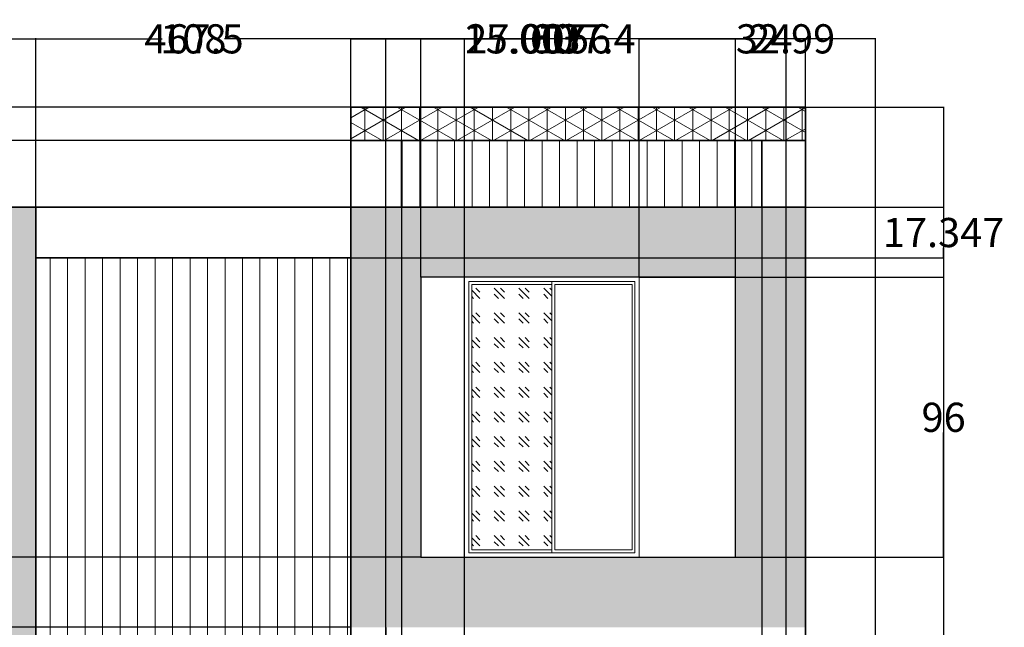
# Model space of a CAD drawing. Units: inches. Extents: x -37 to 519, y -28 to 435.
# Tile 3 of 3: x 182 to 519, y 227 to 435. Entities that reach past the tile are written whole.
import ezdxf

# ---------------------------------------------------------------- set-up
doc = ezdxf.new("R2010")
doc.units = ezdxf.units.IN
doc.header["$MEASUREMENT"] = 0
for name, color, linetype, lineweight in [('A-ANNO-DIMS', 2, 'Continuous', 18), ('A-GLAZ', 4, 'Continuous', 18), ('A-GLAZ-PATT', 9, 'Continuous', 13), ('A-ROOF', 7, 'Continuous', 35), ('A-ROOF-PATT', 8, 'Continuous', 13), ('A-WALL', 7, 'Continuous', 35), ('A-WALL-PATT', 8, 'Continuous', 13), ('A-WALL-TRIM', 7, 'Continuous', 25)]:
    doc.layers.add(name, color=color, linetype=linetype, lineweight=lineweight)
doc.styles.get("Standard").update_dxf_attribs({"font": 'arial.ttf'})
doc.dimstyles.get("Standard").update_dxf_attribs({"dimtxt": 10, "dimasz": 0.18, "dimexe": 0.18, "dimexo": 0.0625, "dimgap": 0.09, "dimtad": 0, "dimtih": 1, "dimtoh": 1, "dimdec": 0, "dimzin": 0, "dimdsep": 46, "dimlunit": 3, "dimtxsty": 'Standard', "dimcen": 0.09, "dimadec": 0, "dimazin": 0, "dimtfac": 1, "dimtdec": 0, "dimtofl": 0, "dimtmove": 0, "dimatfit": 3, "dimfxl": 1, "dimtolj": 1, "dimtzin": 0, "dimarcsym": 0})

# ---------------------------------------------------------------- blocks, each defined once
blk = doc.blocks.new('*D7')
at = {"layer": 'A-ANNO-DIMS', "color": 0, "lineweight": -2, "transparency": 16777216}
for p, q in [((7.62, 97.72), (7.62, 428.56)), ((7.8, 428.38), (224.17, 428.38)), ((474.95, 428.38), (258.57, 428.38)), ((475.13, 97.72), (475.13, 428.56))]:
    blk.add_line(p, q, dxfattribs=at)
at = {"layer": 'A-ANNO-DIMS', "color": 0, "transparency": 16777216}
for points in [[(7.8, 428.41), (7.8, 428.35), (7.62, 428.38)], [(474.95, 428.41), (474.95, 428.35), (475.13, 428.38)]]:
    blk.add_solid(points, dxfattribs=at)
at = {"layer": 'Defpoints', "color": 0, "transparency": 16777216}
for p in [(475.13, 428.38), (7.62, 97.65), (475.13, 97.65)]:
    blk.add_point(p, dxfattribs=at)
at = {"layer": 'A-ANNO-DIMS', "color": 0, "transparency": 16777216, "insert": (241.37, 428.38), "char_height": 10, "attachment_point": 5}
blk.add_mtext('\\A1;467.5', dxfattribs=at)
blk = doc.blocks.new('*D8')
at = {"layer": 'A-ANNO-DIMS', "color": 0, "lineweight": -2, "transparency": 16777216}
for p, q in [((451.19, 404.99), (498.7, 404.99)), ((498.52, 404.81), (498.52, 208.52)), ((498.52, 1.83), (498.52, 198.12)), ((451.19, 1.65), (498.7, 1.65))]:
    blk.add_line(p, q, dxfattribs=at)
at = {"layer": 'A-ANNO-DIMS', "color": 0, "transparency": 16777216}
for points in [[(498.49, 404.81), (498.55, 404.81), (498.52, 404.99)], [(498.49, 1.83), (498.55, 1.83), (498.52, 1.65)]]:
    blk.add_solid(points, dxfattribs=at)
at = {"layer": 'Defpoints', "color": 0, "transparency": 16777216}
for p in [(451.13, 404.99), (498.52, 404.99), (451.13, 1.65)]:
    blk.add_point(p, dxfattribs=at)
at = {"layer": 'A-ANNO-DIMS', "color": 0, "transparency": 16777216, "insert": (498.52, 203.32), "char_height": 10, "attachment_point": 5}
blk.add_mtext('\\A1;403.3', dxfattribs=at)
blk = doc.blocks.new('*D25')
at = {"layer": 'A-ANNO-DIMS', "color": 0, "lineweight": -2, "transparency": 16777216}
for p, q in [((187.19, 370.65), (498.7, 370.65)), ((498.52, 370.47), (498.52, 367.18)), ((498.52, 353.49), (498.52, 356.78)), ((187.19, 353.31), (498.7, 353.31))]:
    blk.add_line(p, q, dxfattribs=at)
at = {"layer": 'A-ANNO-DIMS', "color": 0, "transparency": 16777216}
for points in [[(498.49, 370.47), (498.55, 370.47), (498.52, 370.65)], [(498.49, 353.49), (498.55, 353.49), (498.52, 353.31)]]:
    blk.add_solid(points, dxfattribs=at)
at = {"layer": 'Defpoints', "color": 0, "transparency": 16777216}
for p in [(187.13, 370.65), (498.52, 370.65), (187.13, 353.31)]:
    blk.add_point(p, dxfattribs=at)
at = {"layer": 'A-ANNO-DIMS', "color": 0, "transparency": 16777216, "insert": (498.52, 361.98), "char_height": 10, "attachment_point": 5}
blk.add_mtext('\\A1;17.347', dxfattribs=at)
blk = doc.blocks.new('*D26')
at = {"layer": 'A-ANNO-DIMS', "color": 0, "lineweight": -2, "transparency": 16777216}
for p, q in [((187.13, 353.37), (187.13, 428.56)), ((187.31, 428.38), (230.45, 428.38)), ((294.95, 428.38), (251.8, 428.38)), ((295.13, 353.37), (295.13, 428.56))]:
    blk.add_line(p, q, dxfattribs=at)
at = {"layer": 'A-ANNO-DIMS', "color": 0, "transparency": 16777216}
for points in [[(187.31, 428.41), (187.31, 428.35), (187.13, 428.38)], [(294.95, 428.41), (294.95, 428.35), (295.13, 428.38)]]:
    blk.add_solid(points, dxfattribs=at)
at = {"layer": 'Defpoints', "color": 0, "transparency": 16777216}
for p in [(295.13, 428.38), (187.13, 353.31), (295.13, 353.31)]:
    blk.add_point(p, dxfattribs=at)
at = {"layer": 'A-ANNO-DIMS', "color": 0, "transparency": 16777216, "insert": (241.13, 428.38), "char_height": 10, "attachment_point": 5}
blk.add_mtext('\\A1;108', dxfattribs=at)
blk = doc.blocks.new('*D32')
at = {"layer": 'A-ANNO-DIMS', "color": 0, "lineweight": -2, "transparency": 16777216}
for p, q in [((394.2, 250.65), (498.7, 250.65)), ((498.52, 250.47), (498.52, 195.85)), ((498.52, 130.83), (498.52, 185.46)), ((394.2, 130.65), (498.7, 130.65))]:
    blk.add_line(p, q, dxfattribs=at)
at = {"layer": 'A-ANNO-DIMS', "color": 0, "transparency": 16777216}
for points in [[(498.49, 250.47), (498.55, 250.47), (498.52, 250.65)], [(498.49, 130.83), (498.55, 130.83), (498.52, 130.65)]]:
    blk.add_solid(points, dxfattribs=at)
at = {"layer": 'Defpoints', "color": 0, "transparency": 16777216}
for p in [(394.13, 250.65), (498.52, 250.65), (394.13, 130.65)]:
    blk.add_point(p, dxfattribs=at)
at = {"layer": 'A-ANNO-DIMS', "color": 0, "transparency": 16777216, "insert": (498.52, 190.65), "char_height": 10, "attachment_point": 5}
blk.add_mtext('\\A1;120', dxfattribs=at)
blk = doc.blocks.new('*D33')
at = {"layer": 'A-ANNO-DIMS', "color": 0, "lineweight": -2, "transparency": 16777216}
for p, q in [((319.06, 250.65), (-15.95, 250.65)), ((-15.77, 250.47), (-15.77, 243.76)), ((-15.77, 226.83), (-15.77, 233.54)), ((295.06, 226.65), (-15.95, 226.65))]:
    blk.add_line(p, q, dxfattribs=at)
at = {"layer": 'A-ANNO-DIMS', "color": 0, "transparency": 16777216}
for points in [[(-15.8, 250.47), (-15.74, 250.47), (-15.77, 250.65)], [(-15.8, 226.83), (-15.74, 226.83), (-15.77, 226.65)]]:
    blk.add_solid(points, dxfattribs=at)
at = {"layer": 'Defpoints', "color": 0, "transparency": 16777216}
for p in [(319.13, 250.65), (-15.77, 226.65), (295.13, 226.65)]:
    blk.add_point(p, dxfattribs=at)
at = {"layer": 'A-ANNO-DIMS', "color": 0, "transparency": 16777216, "insert": (-15.77, 238.65), "char_height": 10, "attachment_point": 5}
blk.add_mtext('\\A1;24', dxfattribs=at)
blk = doc.blocks.new('*D34')
at = {"layer": 'A-ANNO-DIMS', "color": 0, "lineweight": -2, "transparency": 16777216}
for p, q in [((394.2, 346.65), (498.7, 346.65)), ((498.52, 346.47), (498.52, 303.85)), ((498.52, 250.83), (498.52, 293.46)), ((394.2, 250.65), (498.7, 250.65))]:
    blk.add_line(p, q, dxfattribs=at)
at = {"layer": 'A-ANNO-DIMS', "color": 0, "transparency": 16777216}
for points in [[(498.49, 346.47), (498.55, 346.47), (498.52, 346.65)], [(498.49, 250.83), (498.55, 250.83), (498.52, 250.65)]]:
    blk.add_solid(points, dxfattribs=at)
at = {"layer": 'Defpoints', "color": 0, "transparency": 16777216}
for p in [(394.13, 346.65), (498.52, 346.65), (394.13, 250.65)]:
    blk.add_point(p, dxfattribs=at)
at = {"layer": 'A-ANNO-DIMS', "color": 0, "transparency": 16777216, "insert": (498.52, 298.65), "char_height": 10, "attachment_point": 5}
blk.add_mtext('\\A1;96', dxfattribs=at)
blk = doc.blocks.new('*D35')
at = {"layer": 'A-ANNO-DIMS', "color": 0, "lineweight": -2, "transparency": 16777216}
for p, q in [((334.13, 346.72), (334.13, 428.56)), ((334.31, 428.38), (356.87, 428.38)), ((393.95, 428.38), (371.4, 428.38)), ((394.13, 346.72), (394.13, 428.56))]:
    blk.add_line(p, q, dxfattribs=at)
at = {"layer": 'A-ANNO-DIMS', "color": 0, "transparency": 16777216}
for points in [[(334.31, 428.41), (334.31, 428.35), (334.13, 428.38)], [(393.95, 428.41), (393.95, 428.35), (394.13, 428.38)]]:
    blk.add_solid(points, dxfattribs=at)
at = {"layer": 'Defpoints', "color": 0, "transparency": 16777216}
for p in [(394.13, 428.38), (334.13, 346.65), (394.13, 346.65)]:
    blk.add_point(p, dxfattribs=at)
at = {"layer": 'A-ANNO-DIMS', "color": 0, "transparency": 16777216, "insert": (364.13, 428.38), "char_height": 10, "attachment_point": 5}
blk.add_mtext('\\A1;60', dxfattribs=at)
blk = doc.blocks.new('*D36')
at = {"layer": 'A-ANNO-DIMS', "color": 0, "lineweight": -2, "transparency": 16777216}
for p, q in [((319.13, 346.72), (319.13, 428.56)), ((319.31, 428.38), (333.95, 428.38)), ((334.13, 346.72), (334.13, 428.56)), ((334.13, 428.38), (334.31, 428.38))]:
    blk.add_line(p, q, dxfattribs=at)
at = {"layer": 'A-ANNO-DIMS', "color": 0, "transparency": 16777216}
for points in [[(319.31, 428.41), (319.31, 428.35), (319.13, 428.38)], [(333.95, 428.41), (333.95, 428.35), (334.13, 428.38)]]:
    blk.add_solid(points, dxfattribs=at)
at = {"layer": 'Defpoints', "color": 0, "transparency": 16777216}
for p in [(334.13, 428.38), (319.13, 346.65), (334.13, 346.65)]:
    blk.add_point(p, dxfattribs=at)
at = {"layer": 'A-ANNO-DIMS', "color": 0, "transparency": 16777216, "insert": (354.69, 428.38), "char_height": 10, "attachment_point": 5}
blk.add_mtext('\\A1;15.007', dxfattribs=at)
blk = doc.blocks.new('*D37')
at = {"layer": 'A-ANNO-DIMS', "color": 0, "lineweight": -2, "transparency": 16777216}
for p, q in [((394.13, 346.72), (394.13, 428.56)), ((394.31, 428.38), (426.95, 428.38)), ((427.13, 346.72), (427.13, 428.56)), ((427.13, 428.38), (427.31, 428.38))]:
    blk.add_line(p, q, dxfattribs=at)
at = {"layer": 'A-ANNO-DIMS', "color": 0, "transparency": 16777216}
for points in [[(394.31, 428.41), (394.31, 428.35), (394.13, 428.38)], [(426.95, 428.41), (426.95, 428.35), (427.13, 428.38)]]:
    blk.add_solid(points, dxfattribs=at)
at = {"layer": 'Defpoints', "color": 0, "transparency": 16777216}
for p in [(427.13, 428.38), (394.13, 346.65), (427.13, 346.65)]:
    blk.add_point(p, dxfattribs=at)
at = {"layer": 'A-ANNO-DIMS', "color": 0, "transparency": 16777216, "insert": (444.28, 428.38), "char_height": 10, "attachment_point": 5}
blk.add_mtext('\\A1;32.99', dxfattribs=at)
blk = doc.blocks.new('*D38')
at = {"layer": 'A-ANNO-DIMS', "color": 0, "lineweight": -2, "transparency": 16777216}
for p, q in [((427.13, 250.72), (427.13, 428.56)), ((427.31, 428.38), (431.81, 428.38)), ((450.95, 428.38), (446.44, 428.38)), ((451.13, 226.72), (451.13, 428.56))]:
    blk.add_line(p, q, dxfattribs=at)
at = {"layer": 'A-ANNO-DIMS', "color": 0, "transparency": 16777216}
for points in [[(427.31, 428.41), (427.31, 428.35), (427.13, 428.38)], [(450.95, 428.41), (450.95, 428.35), (451.13, 428.38)]]:
    blk.add_solid(points, dxfattribs=at)
at = {"layer": 'Defpoints', "color": 0, "transparency": 16777216}
for p in [(451.13, 428.38), (427.13, 250.65), (451.13, 226.65)]:
    blk.add_point(p, dxfattribs=at)
at = {"layer": 'A-ANNO-DIMS', "color": 0, "transparency": 16777216, "insert": (439.13, 428.38), "char_height": 10, "attachment_point": 5}
blk.add_mtext('\\A1;24', dxfattribs=at)
blk = doc.blocks.new('*D39')
at = {"layer": 'A-ANNO-DIMS', "color": 0, "lineweight": -2, "transparency": 16777216}
for p, q in [((295.13, 405.05), (295.13, 428.56)), ((295.31, 428.38), (362.46, 428.38)), ((450.95, 428.38), (383.79, 428.38)), ((451.13, 405.05), (451.13, 428.56))]:
    blk.add_line(p, q, dxfattribs=at)
at = {"layer": 'A-ANNO-DIMS', "color": 0, "transparency": 16777216}
for points in [[(295.31, 428.41), (295.31, 428.35), (295.13, 428.38)], [(450.95, 428.41), (450.95, 428.35), (451.13, 428.38)]]:
    blk.add_solid(points, dxfattribs=at)
at = {"layer": 'Defpoints', "color": 0, "transparency": 16777216}
for p in [(451.13, 428.38), (295.13, 404.99), (451.13, 404.99)]:
    blk.add_point(p, dxfattribs=at)
at = {"layer": 'A-ANNO-DIMS', "color": 0, "transparency": 16777216, "insert": (373.13, 428.38), "char_height": 10, "attachment_point": 5}
blk.add_mtext('\\A1;156', dxfattribs=at)
blk = doc.blocks.new('*D40')
at = {"layer": 'A-ANNO-DIMS', "color": 0, "lineweight": -2, "transparency": 16777216}
for p, q in [((295.13, 393.45), (295.13, -21.92)), ((312.5, 393.45), (312.5, -21.92)), ((295.31, -21.74), (312.32, -21.74)), ((312.5, -21.74), (312.68, -21.74))]:
    blk.add_line(p, q, dxfattribs=at)
at = {"layer": 'A-ANNO-DIMS', "color": 0, "transparency": 16777216}
for points in [[(295.31, -21.71), (295.31, -21.77), (295.13, -21.74)], [(312.32, -21.71), (312.32, -21.77), (312.5, -21.74)]]:
    blk.add_solid(points, dxfattribs=at)
at = {"layer": 'Defpoints', "color": 0, "transparency": 16777216}
for p in [(295.13, 393.51), (312.5, 393.51), (312.5, -21.74)]:
    blk.add_point(p, dxfattribs=at)
at = {"layer": 'A-ANNO-DIMS', "color": 0, "transparency": 16777216, "insert": (333.06, -21.74), "char_height": 10, "attachment_point": 5}
blk.add_mtext('\\A1;17.376', dxfattribs=at)
blk = doc.blocks.new('*D41')
at = {"layer": 'A-ANNO-DIMS', "color": 0, "lineweight": -2, "transparency": 16777216}
for p, q in [((436.2, 393.45), (436.2, -21.92)), ((451.13, 393.45), (451.13, -21.92)), ((436.38, -21.74), (450.95, -21.74)), ((451.13, -21.74), (451.31, -21.74))]:
    blk.add_line(p, q, dxfattribs=at)
at = {"layer": 'A-ANNO-DIMS', "color": 0, "transparency": 16777216}
for points in [[(436.38, -21.71), (436.38, -21.77), (436.2, -21.74)], [(450.95, -21.71), (450.95, -21.77), (451.13, -21.74)]]:
    blk.add_solid(points, dxfattribs=at)
at = {"layer": 'Defpoints', "color": 0, "transparency": 16777216}
for p in [(436.2, 393.51), (451.13, 393.51), (451.13, -21.74)]:
    blk.add_point(p, dxfattribs=at)
at = {"layer": 'A-ANNO-DIMS', "color": 0, "transparency": 16777216, "insert": (471.72, -21.74), "char_height": 10, "attachment_point": 5}
blk.add_mtext('\\A1;14.925', dxfattribs=at)
blk = doc.blocks.new('*D42')
at = {"layer": 'A-ANNO-DIMS', "color": 0, "lineweight": -2, "transparency": 16777216}
for p, q in [((312.44, 393.51), (-15.95, 393.51)), ((-15.77, 393.33), (-15.77, 387.28)), ((-15.77, 370.83), (-15.77, 376.89)), ((312.44, 370.65), (-15.95, 370.65))]:
    blk.add_line(p, q, dxfattribs=at)
at = {"layer": 'A-ANNO-DIMS', "color": 0, "transparency": 16777216}
for points in [[(-15.8, 393.33), (-15.74, 393.33), (-15.77, 393.51)], [(-15.8, 370.83), (-15.74, 370.83), (-15.77, 370.65)]]:
    blk.add_solid(points, dxfattribs=at)
at = {"layer": 'Defpoints', "color": 0, "transparency": 16777216}
for p in [(-15.77, 393.51), (312.5, 393.51), (312.5, 370.65)]:
    blk.add_point(p, dxfattribs=at)
at = {"layer": 'A-ANNO-DIMS', "color": 0, "transparency": 16777216, "insert": (-15.77, 382.08), "char_height": 10, "attachment_point": 5}
blk.add_mtext('\\A1;22.856', dxfattribs=at)
blk = doc.blocks.new('*D43')
at = {"layer": 'A-ANNO-DIMS', "color": 0, "lineweight": -2, "transparency": 16777216}
for p, q in [((295.06, 404.99), (-15.95, 404.99)), ((-15.77, 404.81), (-15.77, 404.44)), ((295.06, 393.51), (-15.95, 393.51)), ((-15.77, 393.69), (-15.77, 394.05))]:
    blk.add_line(p, q, dxfattribs=at)
at = {"layer": 'A-ANNO-DIMS', "color": 0, "transparency": 16777216}
for points in [[(-15.8, 404.81), (-15.74, 404.81), (-15.77, 404.99)], [(-15.8, 393.69), (-15.74, 393.69), (-15.77, 393.51)]]:
    blk.add_solid(points, dxfattribs=at)
at = {"layer": 'Defpoints', "color": 0, "transparency": 16777216}
for p in [(-15.77, 404.99), (295.13, 404.99), (295.13, 393.51)]:
    blk.add_point(p, dxfattribs=at)
at = {"layer": 'A-ANNO-DIMS', "color": 0, "transparency": 16777216, "insert": (-15.77, 399.25), "char_height": 10, "attachment_point": 5}
blk.add_mtext('\\A1;11.48', dxfattribs=at)
blk = doc.blocks.new('*D44')
at = {"layer": 'A-ANNO-DIMS', "color": 0, "lineweight": -2, "transparency": 16777216}
for p, q in [((307.13, 220.19), (307.13, 428.56)), ((307.31, 428.38), (359.36, 428.38)), ((444.36, 428.38), (392.3, 428.38)), ((444.54, 220.19), (444.54, 428.56))]:
    blk.add_line(p, q, dxfattribs=at)
at = {"layer": 'A-ANNO-DIMS', "color": 0, "transparency": 16777216}
for points in [[(307.31, 428.41), (307.31, 428.35), (307.13, 428.38)], [(444.36, 428.41), (444.36, 428.35), (444.54, 428.38)]]:
    blk.add_solid(points, dxfattribs=at)
at = {"layer": 'Defpoints', "color": 0, "transparency": 16777216}
for p in [(444.54, 428.38), (307.13, 220.13), (444.54, 220.13)]:
    blk.add_point(p, dxfattribs=at)
at = {"layer": 'A-ANNO-DIMS', "color": 0, "transparency": 16777216, "insert": (375.83, 428.38), "char_height": 10, "attachment_point": 5}
blk.add_mtext('\\A1;137.4', dxfattribs=at)
blk = doc.blocks.new('*D47')
at = {"layer": 'A-ANNO-DIMS', "color": 0, "lineweight": -2, "transparency": 16777216}
for p, q in [((307.13, 130.72), (307.13, 428.56)), ((307.31, 428.38), (333.95, 428.38)), ((334.13, 130.72), (334.13, 428.56)), ((334.13, 428.38), (334.31, 428.38))]:
    blk.add_line(p, q, dxfattribs=at)
at = {"layer": 'A-ANNO-DIMS', "color": 0, "transparency": 16777216}
for points in [[(307.31, 428.41), (307.31, 428.35), (307.13, 428.38)], [(333.95, 428.41), (333.95, 428.35), (334.13, 428.38)]]:
    blk.add_solid(points, dxfattribs=at)
at = {"layer": 'Defpoints', "color": 0, "transparency": 16777216}
for p in [(334.13, 428.38), (307.13, 130.65), (334.13, 130.65)]:
    blk.add_point(p, dxfattribs=at)
at = {"layer": 'A-ANNO-DIMS', "color": 0, "transparency": 16777216, "insert": (355.25, 428.38), "char_height": 10, "attachment_point": 5}
blk.add_mtext('\\A1;27.007', dxfattribs=at)
blk = doc.blocks.new('*D48')
at = {"layer": 'A-ANNO-DIMS', "color": 0, "lineweight": -2, "transparency": 16777216}
for p, q in [((295.13, 226.59), (295.13, -21.92)), ((307.13, 226.59), (307.13, -21.92)), ((295.31, -21.74), (306.95, -21.74)), ((307.13, -21.74), (307.31, -21.74))]:
    blk.add_line(p, q, dxfattribs=at)
at = {"layer": 'A-ANNO-DIMS', "color": 0, "transparency": 16777216}
for points in [[(295.31, -21.71), (295.31, -21.77), (295.13, -21.74)], [(306.95, -21.71), (306.95, -21.77), (307.13, -21.74)]]:
    blk.add_solid(points, dxfattribs=at)
at = {"layer": 'Defpoints', "color": 0, "transparency": 16777216}
for p in [(295.13, 226.65), (307.13, 226.65), (307.13, -21.74)]:
    blk.add_point(p, dxfattribs=at)
at = {"layer": 'A-ANNO-DIMS', "color": 0, "transparency": 16777216, "insert": (314.04, -21.74), "char_height": 10, "attachment_point": 5}
blk.add_mtext('\\A1;12', dxfattribs=at)

msp = doc.modelspace()

# ---------------------------------------------------------------- hatches: boundary and pattern name
at = {"layer": 'A-GLAZ-PATT'}
h = msp.add_hatch(dxfattribs=at)
h.set_pattern_fill('GOST_GLASS', color=256, angle=90)
h.set_pattern_definition([(135, (0, 0), (5e-16, 8.48528), [5, -7]), (135, (1e-16, 2.1213), (5e-16, 8.48528), [2, -10]), (135, (-2.1213, 1e-16), (5e-16, 8.48528), [2, -10])])
h.paths.add_polyline_path([(364.1341, 344.153), (336.6341, 344.153), (336.6341, 253.153), (364.1341, 253.153)])
at = {"layer": 'A-ROOF-PATT'}
h = msp.add_hatch(dxfattribs=at)
h.set_pattern_fill('NET3', color=256, scale=50, angle=90)
h.paths.add_polyline_path([(451.1272, 404.9893), (295.1272, 404.9893), (295.1272, 393.509), (451.1272, 393.509)])
h = msp.add_hatch(dxfattribs=at)
h.set_pattern_fill('_USER', color=256, scale=6, angle=90, pattern_type=0)
h.set_pattern_definition([(90, (0.779, 0), (-6, 4e-16), [])])
h.paths.add_polyline_path([(436.2023, 393.509), (312.5031, 393.509), (312.5031, 370.653), (436.2023, 370.653)])
at = {"layer": 'A-WALL-PATT'}
h = msp.add_hatch(color=256, dxfattribs=at)
h.dxf.hatch_style = 1
h.paths.add_polyline_path([(451.1272, 370.653), (295.1272, 370.653), (295.1272, 226.653), (451.1272, 226.653)])
h.paths.add_polyline_path([(319.1272, 346.653), (427.1272, 346.653), (427.1272, 250.653), (319.1272, 250.653)], flags=16)
h.paths.add_polyline_path([(334.1341, 346.653), (394.1341, 346.653), (394.1341, 250.653), (334.1341, 250.653)], flags=0)
h.paths.add_polyline_path([(335.6341, 345.153), (364.1341, 345.153), (392.6341, 345.153), (392.6341, 252.153), (364.1341, 252.153), (335.6341, 252.153)], flags=0)
h.paths.add_polyline_path([(336.6341, 344.153), (364.1341, 344.153), (364.1341, 253.153), (336.6341, 253.153)], flags=0)
h.paths.add_polyline_path([(365.1341, 344.153), (391.6341, 344.153), (391.6341, 253.153), (365.1341, 253.153)], flags=0)
h.paths.add_polyline_path([(187.1272, 370.653), (175.1272, 370.653), (175.1272, 256.7765), (31.1272, 256.7765), (31.1272, 97.653), (55.1272, 97.653), (55.1272, 106.653), (175.1272, 106.653), (175.1272, 97.653), (187.1272, 97.653)])
h.paths.add_polyline_path([(175.1272, 208.7765), (175.1272, 130.653), (55.1272, 130.653), (55.1272, 208.7765)], flags=16)
h.paths.add_polyline_path([(142.1341, 208.653), (142.1341, 130.653), (82.1341, 130.653), (82.1341, 208.653)], flags=0)
h.paths.add_polyline_path([(112.1341, 207.153), (140.6341, 207.153), (140.6341, 132.153), (112.1341, 132.153), (83.6341, 132.153), (83.6341, 207.153)], flags=0)
h.paths.add_polyline_path([(112.1341, 133.153), (84.6341, 133.153), (84.6341, 206.153), (112.1341, 206.153)], flags=0)
h.paths.add_polyline_path([(139.6341, 206.153), (139.6341, 133.153), (113.1341, 133.153), (113.1341, 206.153)], flags=0)
h.paths.add_polyline_path([(187.1272, 88.653), (175.1272, 88.653), (175.1272, 10.653), (187.1272, 10.653)])
h.paths.add_polyline_path([(307.1272, 88.653), (295.1272, 88.653), (295.1272, 10.653), (307.1272, 10.653)])
h.paths.add_polyline_path([(451.1272, 88.653), (427.1272, 88.653), (427.1272, 10.653), (451.1272, 10.653)])
h = msp.add_hatch(dxfattribs=at)
h.set_pattern_fill('_USER', color=256, scale=6, angle=90, pattern_type=0)
h.set_pattern_definition([(90, (0, 0), (-6, 4e-16), [])])
h.paths.add_polyline_path([(295.1272, 353.3062), (187.1272, 353.3062), (187.1272, 130.653), (295.1272, 130.653)])

# ---------------------------------------------------------------- linework, layer by layer
at = {"layer": 'A-GLAZ'}
for p, q in [((364.1341, 345.153), (335.6341, 345.153)), ((335.6341, 345.153), (335.6341, 252.153)), ((364.1341, 345.153), (335.6341, 345.153)), ((335.6341, 345.153), (335.6341, 252.153)), ((364.1341, 252.153), (364.1341, 345.153)), ((392.6341, 345.153), (364.1341, 345.153)), ((364.1341, 252.153), (364.1341, 345.153)), ((392.6341, 345.153), (364.1341, 345.153)), ((392.6341, 252.153), (392.6341, 345.153)), ((392.6341, 252.153), (392.6341, 345.153)), ((335.6341, 252.153), (364.1341, 252.153)), ((335.6341, 252.153), (364.1341, 252.153)), ((364.1341, 252.153), (392.6341, 252.153)), ((364.1341, 252.153), (392.6341, 252.153))]:
    msp.add_line(p, q, dxfattribs=at)
msp.add_lwpolyline([(394.1341, 250.653), (394.1341, 346.653), (334.1341, 346.653), (334.1341, 250.653)], close=True, dxfattribs=at)
msp.add_lwpolyline([(394.1341, 250.653), (394.1341, 346.653), (334.1341, 346.653), (334.1341, 250.653)], close=True, dxfattribs=at)
for points in [[(364.1341, 344.153), (336.6341, 344.153), (336.6341, 253.153), (364.1341, 253.153)], [(364.1341, 344.153), (336.6341, 344.153), (336.6341, 253.153), (364.1341, 253.153)], [(365.1341, 344.153), (365.1341, 253.153), (391.6341, 253.153), (391.6341, 344.153), (365.1341, 344.153)], [(365.1341, 344.153), (365.1341, 253.153), (391.6341, 253.153), (391.6341, 344.153), (365.1341, 344.153)]]:
    msp.add_lwpolyline(points, dxfattribs=at)
at = {"layer": 'A-ROOF'}
for points in [[(295.1272, 393.509), (451.1272, 393.509), (451.1272, 404.9893), (295.1272, 404.9893)], [(312.5031, 370.653), (436.2023, 370.653), (436.2023, 393.509), (312.5031, 393.509)]]:
    msp.add_lwpolyline(points, close=True, dxfattribs=at)
at = {"layer": 'A-WALL'}
for p, q in [((187.1272, 370.653), (81.851, 370.653)), ((187.1272, 370.653), (187.1272, 10.653)), ((451.1272, 370.653), (295.1272, 370.653)), ((295.1272, 370.653), (295.1272, 10.653)), ((451.1272, 97.653), (451.1272, 370.653)), ((187.1272, 353.3062), (295.1272, 353.3062))]:
    msp.add_line(p, q, dxfattribs=at)
at = {"layer": 'A-WALL-TRIM'}
for p, q in [((427.1272, 346.653), (319.1272, 346.653)), ((319.1272, 346.653), (319.1272, 250.653)), ((427.1272, 250.653), (427.1272, 346.653)), ((319.1272, 250.653), (427.1272, 250.653))]:
    msp.add_line(p, q, dxfattribs=at)

# ---------------------------------------------------------------- dimensions: what is measured, and where the dimension line sits
at = {"layer": 'A-ANNO-DIMS'}
for base, p1, p2, override, picture, middle in [((475.1272, 428.3793), (7.6202, 97.653), (475.1272, 97.653), {"dimdec": 1, "dimlfac": 1, "dimrnd": 0, "dimzin": 0, "dimdsep": 46, "dimlunit": 2}, '*D7', (241.3737, 428.3793)), ((295.1272, 428.3793), (187.1272, 353.3062), (295.1272, 353.3062), {"dimdec": 0, "dimlfac": 1, "dimrnd": 0, "dimzin": 0, "dimdsep": 46, "dimlunit": 2}, '*D26', (241.1272, 428.3793)), ((451.1272, 428.3793), (295.1272, 404.9893), (451.1272, 404.9893), {"dimdec": 0, "dimlfac": 1, "dimrnd": 0, "dimzin": 0, "dimdsep": 46, "dimlunit": 2}, '*D39', (373.1272, 428.3793)), ((444.5372, 428.3793), (307.1272, 220.1322), (444.5372, 220.1322), {"dimdec": 1, "dimlfac": 1, "dimrnd": 0, "dimzin": 0, "dimdsep": 46, "dimlunit": 2}, '*D44', (375.8322, 428.3793)), ((334.1341, 428.3793), (307.1272, 130.653), (334.1341, 130.653), {"dimdec": 3, "dimlfac": 1, "dimrnd": 0, "dimzin": 0, "dimdsep": 46, "dimlunit": 2}, '*D47', (355.2465, 428.3793)), ((334.1341, 428.3793), (319.1272, 346.653), (334.1341, 346.653), {"dimdec": 3, "dimlfac": 1, "dimrnd": 0, "dimzin": 0, "dimdsep": 46, "dimlunit": 2}, '*D36', (354.6906, 428.3793)), ((394.1341, 428.3793), (334.1341, 346.653), (394.1341, 346.653), {"dimdec": 0, "dimlfac": 1, "dimrnd": 0, "dimzin": 0, "dimdsep": 46, "dimlunit": 2}, '*D35', (364.1341, 428.3793)), ((427.1272, 428.3793), (394.1341, 346.653), (427.1272, 346.653), {"dimdec": 2, "dimlfac": 1, "dimrnd": 0, "dimzin": 0, "dimdsep": 46, "dimlunit": 2}, '*D37', (444.2765, 428.3793)), ((451.1272, 428.3793), (427.1272, 250.653), (451.1272, 226.653), {"dimdec": 0, "dimlfac": 1, "dimrnd": 0, "dimzin": 0, "dimdsep": 46, "dimlunit": 2}, '*D38', (439.1272, 428.3793)), ((312.5031, -21.737), (295.1272, 393.509), (312.5031, 393.509), {"dimdec": 3, "dimlfac": 1, "dimrnd": 0, "dimzin": 0, "dimdsep": 46, "dimlunit": 2}, '*D40', (333.0562, -21.737)), ((451.1272, -21.737), (436.2023, 393.509), (451.1272, 393.509), {"dimdec": 3, "dimlfac": 1, "dimrnd": 0, "dimzin": 0, "dimdsep": 46, "dimlunit": 2}, '*D41', (471.7213, -21.737)), ((307.1272, -21.737), (295.1272, 226.653), (307.1272, 226.653), {"dimdec": 0, "dimlfac": 1, "dimrnd": 0, "dimzin": 0, "dimdsep": 46, "dimlunit": 2}, '*D48', (314.0378, -21.737))]:
    dim = msp.add_linear_dim(base=base, p1=p1, p2=p2, dimstyle='Standard', override=override, dxfattribs=at)
    dim.commit()
    dim.dimension.update_dxf_attribs({"geometry": picture, "text_midpoint": middle})
for base, p1, p2, override, picture, middle in [((-15.7698, 404.9893), (295.1272, 393.509), (295.1272, 404.9893), {"dimdec": 2, "dimlfac": 1, "dimrnd": 0, "dimzin": 0, "dimdsep": 46, "dimlunit": 2}, '*D43', (-15.7698, 399.2491)), ((498.5172, 404.9893), (451.1272, 1.653), (451.1272, 404.9893), {"dimdec": 1, "dimlfac": 1, "dimrnd": 0, "dimzin": 0, "dimdsep": 46, "dimlunit": 2}, '*D8', (498.5172, 203.3211)), ((-15.7698, 393.509), (312.5031, 370.653), (312.5031, 393.509), {"dimdec": 3, "dimlfac": 1, "dimrnd": 0, "dimzin": 0, "dimdsep": 46, "dimlunit": 2}, '*D42', (-15.7698, 382.081)), ((498.5172, 370.653), (187.1272, 353.3062), (187.1272, 370.653), {"dimdec": 3, "dimlfac": 1, "dimrnd": 0, "dimzin": 0, "dimdsep": 46, "dimlunit": 2}, '*D25', (498.5172, 361.9796)), ((498.5172, 346.653), (394.1341, 250.653), (394.1341, 346.653), {"dimdec": 0, "dimlfac": 1, "dimrnd": 0, "dimzin": 0, "dimdsep": 46, "dimlunit": 2}, '*D34', (498.5172, 298.653)), ((-15.7698, 226.653), (319.1272, 250.653), (295.1272, 226.653), {"dimdec": 0, "dimlfac": 1, "dimrnd": 0, "dimzin": 0, "dimdsep": 46, "dimlunit": 2}, '*D33', (-15.7698, 238.653)), ((498.5172, 250.653), (394.1341, 130.653), (394.1341, 250.653), {"dimdec": 0, "dimlfac": 1, "dimrnd": 0, "dimzin": 0, "dimdsep": 46, "dimlunit": 2}, '*D32', (498.5172, 190.653))]:
    dim = msp.add_linear_dim(base=base, p1=p1, p2=p2, angle=90, dimstyle='Standard', override=override, dxfattribs=at)
    dim.commit()
    dim.dimension.update_dxf_attribs({"geometry": picture, "text_midpoint": middle})

doc.saveas('drawing.dxf')
